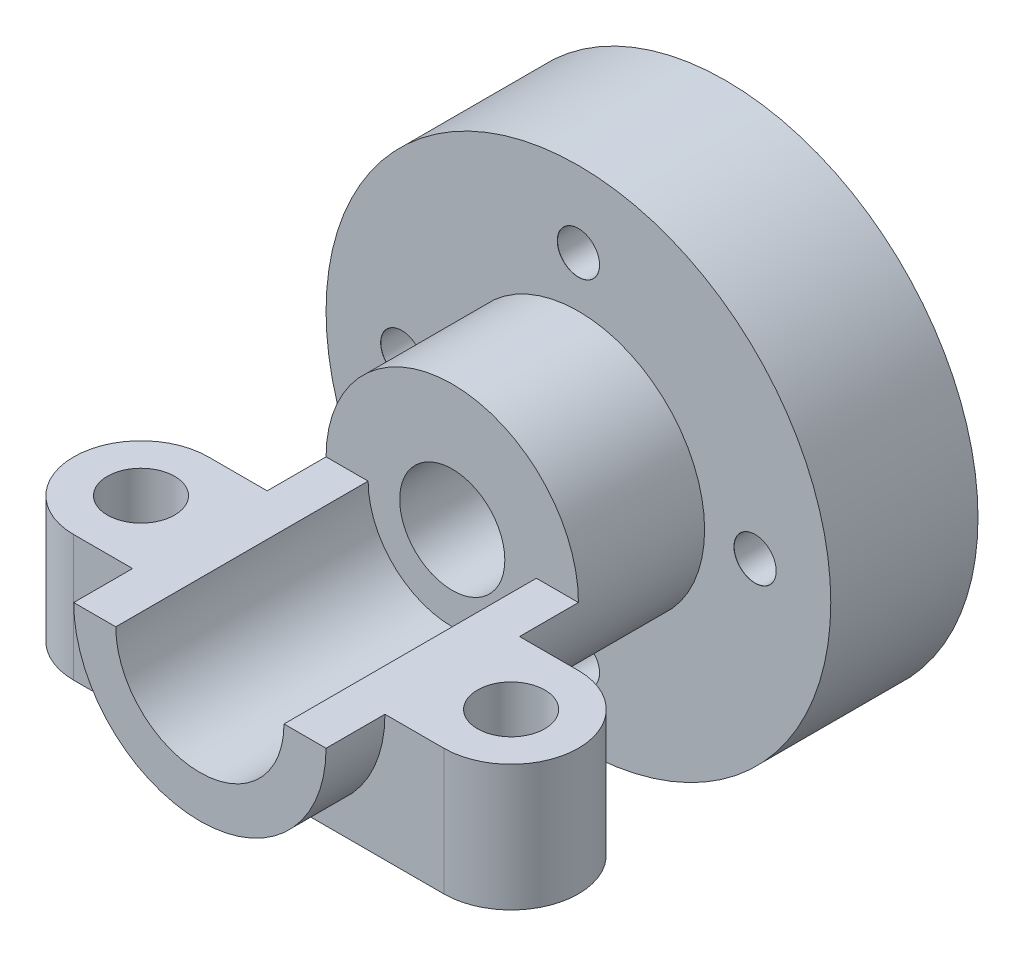
ISO-10303-21;
HEADER;
FILE_DESCRIPTION(('STEP AP214'),'2;1');
FILE_NAME('part.step','',(''),(''),'','','');
FILE_SCHEMA(('AUTOMOTIVE_DESIGN { 1 0 10303 214 1 1 1 1 }'));
ENDSEC;
DATA;
#1=APPLICATION_CONTEXT('core data for automotive mechanical design processes');
#2=APPLICATION_PROTOCOL_DEFINITION('international standard','automotive_design',2000,#1);
#3=PRODUCT_CONTEXT('',#1,'mechanical');
#4=PRODUCT('Part','Part','',(#3));
#5=PRODUCT_RELATED_PRODUCT_CATEGORY('part','',(#4));
#6=PRODUCT_DEFINITION_FORMATION('','',#4);
#7=PRODUCT_DEFINITION_CONTEXT('part definition',#1,'design');
#8=PRODUCT_DEFINITION('design','',#6,#7);
#9=PRODUCT_DEFINITION_SHAPE('','',#8);
#10=(LENGTH_UNIT() NAMED_UNIT(*) SI_UNIT(.MILLI.,.METRE.));
#11=(NAMED_UNIT(*) PLANE_ANGLE_UNIT() SI_UNIT($,.RADIAN.));
#12=(NAMED_UNIT(*) SI_UNIT($,.STERADIAN.) SOLID_ANGLE_UNIT());
#13=UNCERTAINTY_MEASURE_WITH_UNIT(LENGTH_MEASURE(1.E-05),#10,'distance_accuracy_value','');
#14=(GEOMETRIC_REPRESENTATION_CONTEXT(3) GLOBAL_UNCERTAINTY_ASSIGNED_CONTEXT((#13)) GLOBAL_UNIT_ASSIGNED_CONTEXT((#10,
#11,#12)) REPRESENTATION_CONTEXT('',''));
#15=CARTESIAN_POINT('',(0.,0.,0.));
#16=DIRECTION('',(0.,0.,1.));
#17=DIRECTION('',(1.,0.,0.));
#18=AXIS2_PLACEMENT_3D('',#15,#16,#17);
#19=CARTESIAN_POINT('',(-30.,0.,125.));
#20=DIRECTION('',(0.,-1.,0.));
#21=DIRECTION('',(0.,0.,-1.));
#22=AXIS2_PLACEMENT_3D('',#19,#20,#21);
#23=PLANE('',#22);
#24=CARTESIAN_POINT('',(44.,0.,95.));
#25=DIRECTION('',(0.,1.,0.));
#26=DIRECTION('',(0.,0.,1.));
#27=AXIS2_PLACEMENT_3D('',#24,#25,#26);
#28=CIRCLE('',#27,8.);
#29=CARTESIAN_POINT('',(44.,0.,103.));
#30=VERTEX_POINT('',#29);
#31=EDGE_CURVE('E317',#30,#30,#28,.T.);
#32=ORIENTED_EDGE('',*,*,#31,.F.);
#33=EDGE_LOOP('',(#32));
#34=FACE_BOUND('',#33,.T.);
#35=DIRECTION('',(-1.,0.,0.));
#36=VECTOR('',#35,1.);
#37=CARTESIAN_POINT('',(20.,0.,65.));
#38=LINE('',#37,#36);
#39=CARTESIAN_POINT('',(30.,0.,65.));
#40=VERTEX_POINT('',#39);
#41=CARTESIAN_POINT('',(20.,0.,65.));
#42=VERTEX_POINT('',#41);
#43=EDGE_CURVE('E240',#40,#42,#38,.T.);
#44=ORIENTED_EDGE('',*,*,#43,.T.);
#45=DIRECTION('',(0.,0.,-1.));
#46=VECTOR('',#45,1.);
#47=CARTESIAN_POINT('',(20.,0.,125.));
#48=LINE('',#47,#46);
#49=CARTESIAN_POINT('',(20.,0.,125.));
#50=VERTEX_POINT('',#49);
#51=EDGE_CURVE('E63',#50,#42,#48,.T.);
#52=ORIENTED_EDGE('',*,*,#51,.F.);
#53=DIRECTION('',(-1.,0.,0.));
#54=VECTOR('',#53,1.);
#55=CARTESIAN_POINT('',(20.,0.,125.));
#56=LINE('',#55,#54);
#57=CARTESIAN_POINT('',(30.,0.,125.));
#58=VERTEX_POINT('',#57);
#59=EDGE_CURVE('E241',#58,#50,#56,.T.);
#60=ORIENTED_EDGE('',*,*,#59,.F.);
#61=DIRECTION('',(0.,0.,-1.));
#62=VECTOR('',#61,1.);
#63=CARTESIAN_POINT('',(30.,0.,125.));
#64=LINE('',#63,#62);
#65=CARTESIAN_POINT('',(30.,0.,111.));
#66=VERTEX_POINT('',#65);
#67=EDGE_CURVE('E253',#58,#66,#64,.T.);
#68=ORIENTED_EDGE('',*,*,#67,.T.);
#69=DIRECTION('',(1.,0.,0.));
#70=VECTOR('',#69,1.);
#71=CARTESIAN_POINT('',(44.,0.,111.));
#72=LINE('',#71,#70);
#73=CARTESIAN_POINT('',(44.,0.,111.));
#74=VERTEX_POINT('',#73);
#75=EDGE_CURVE('E57',#66,#74,#72,.T.);
#76=ORIENTED_EDGE('',*,*,#75,.T.);
#77=CARTESIAN_POINT('',(44.,0.,95.));
#78=DIRECTION('',(0.,1.,0.));
#79=DIRECTION('',(0.,0.,-1.));
#80=AXIS2_PLACEMENT_3D('',#77,#78,#79);
#81=CIRCLE('',#80,16.);
#82=CARTESIAN_POINT('',(44.,0.,79.));
#83=VERTEX_POINT('',#82);
#84=EDGE_CURVE('E174',#74,#83,#81,.T.);
#85=ORIENTED_EDGE('',*,*,#84,.T.);
#86=DIRECTION('',(-1.,0.,0.));
#87=VECTOR('',#86,1.);
#88=CARTESIAN_POINT('',(-44.,0.,79.));
#89=LINE('',#88,#87);
#90=CARTESIAN_POINT('',(30.,0.,79.));
#91=VERTEX_POINT('',#90);
#92=EDGE_CURVE('E154',#83,#91,#89,.T.);
#93=ORIENTED_EDGE('',*,*,#92,.T.);
#94=EDGE_CURVE('E249',#91,#40,#64,.T.);
#95=ORIENTED_EDGE('',*,*,#94,.T.);
#96=EDGE_LOOP('',(#44,#52,#60,#68,#76,#85,#93,#95));
#97=FACE_BOUND('',#96,.T.);
#98=ADVANCED_FACE('F39',(#34,#97),#23,.F.);
#99=CARTESIAN_POINT('',(0.,0.,65.));
#100=DIRECTION('',(0.,0.,-1.));
#101=DIRECTION('',(-1.,0.,0.));
#102=AXIS2_PLACEMENT_3D('',#99,#100,#101);
#103=CYLINDRICAL_SURFACE('',#102,30.);
#104=DIRECTION('',(0.,0.,-1.));
#105=VECTOR('',#104,1.);
#106=CARTESIAN_POINT('',(-30.,0.,125.));
#107=LINE('',#106,#105);
#108=CARTESIAN_POINT('',(-30.,0.,125.));
#109=VERTEX_POINT('',#108);
#110=CARTESIAN_POINT('',(-30.,0.,111.));
#111=VERTEX_POINT('',#110);
#112=EDGE_CURVE('E254',#109,#111,#107,.T.);
#113=ORIENTED_EDGE('',*,*,#112,.T.);
#114=CARTESIAN_POINT('',(0.,0.,111.));
#115=DIRECTION('',(0.,0.,1.));
#116=DIRECTION('',(1.,0.,0.));
#117=AXIS2_PLACEMENT_3D('',#114,#115,#116);
#118=CIRCLE('',#117,30.);
#119=CARTESIAN_POINT('',(0.,-30.,111.));
#120=VERTEX_POINT('',#119);
#121=EDGE_CURVE('E185',#111,#120,#118,.T.);
#122=ORIENTED_EDGE('',*,*,#121,.T.);
#123=EDGE_CURVE('E180',#120,#66,#118,.T.);
#124=ORIENTED_EDGE('',*,*,#123,.T.);
#125=ORIENTED_EDGE('',*,*,#67,.F.);
#126=CARTESIAN_POINT('',(0.,0.,125.));
#127=DIRECTION('',(0.,0.,1.));
#128=DIRECTION('',(1.,0.,0.));
#129=AXIS2_PLACEMENT_3D('',#126,#127,#128);
#130=CIRCLE('',#129,30.);
#131=EDGE_CURVE('E239',#109,#58,#130,.T.);
#132=ORIENTED_EDGE('',*,*,#131,.F.);
#133=EDGE_LOOP('',(#113,#122,#124,#125,#132));
#134=FACE_BOUND('',#133,.T.);
#135=ADVANCED_FACE('F282',(#134),#103,.T.);
#136=CARTESIAN_POINT('',(0.,0.,-0.001000000000001));
#137=DIRECTION('',(0.,0.,1.));
#138=DIRECTION('',(1.,0.,0.));
#139=AXIS2_PLACEMENT_3D('',#136,#137,#138);
#140=CYLINDRICAL_SURFACE('',#139,12.5);
#141=CARTESIAN_POINT('',(0.,0.,65.));
#142=DIRECTION('',(0.,0.,1.));
#143=DIRECTION('',(1.,0.,0.));
#144=AXIS2_PLACEMENT_3D('',#141,#142,#143);
#145=CIRCLE('',#144,12.5);
#146=CARTESIAN_POINT('',(12.5,0.,65.));
#147=VERTEX_POINT('',#146);
#148=EDGE_CURVE('E228',#147,#147,#145,.T.);
#149=ORIENTED_EDGE('',*,*,#148,.T.);
#150=EDGE_LOOP('',(#149));
#151=FACE_BOUND('',#150,.T.);
#152=CARTESIAN_POINT('',(0.,0.,15.));
#153=DIRECTION('',(0.,0.,-1.));
#154=DIRECTION('',(-1.,0.,0.));
#155=AXIS2_PLACEMENT_3D('',#152,#153,#154);
#156=CIRCLE('',#155,12.5);
#157=CARTESIAN_POINT('',(-12.5,0.,15.));
#158=VERTEX_POINT('',#157);
#159=EDGE_CURVE('E43',#158,#158,#156,.F.);
#160=ORIENTED_EDGE('',*,*,#159,.F.);
#161=EDGE_LOOP('',(#160));
#162=FACE_BOUND('',#161,.T.);
#163=ADVANCED_FACE('F296',(#151,#162),#140,.F.);
#164=CARTESIAN_POINT('',(0.,0.,35.));
#165=DIRECTION('',(0.,0.,-1.));
#166=DIRECTION('',(-1.,0.,0.));
#167=AXIS2_PLACEMENT_3D('',#164,#165,#166);
#168=CYLINDRICAL_SURFACE('',#167,60.);
#169=CARTESIAN_POINT('',(0.,0.,35.));
#170=DIRECTION('',(0.,0.,1.));
#171=DIRECTION('',(1.,0.,0.));
#172=AXIS2_PLACEMENT_3D('',#169,#170,#171);
#173=CIRCLE('',#172,60.);
#174=CARTESIAN_POINT('',(60.,0.,35.));
#175=VERTEX_POINT('',#174);
#176=EDGE_CURVE('E48',#175,#175,#173,.T.);
#177=ORIENTED_EDGE('',*,*,#176,.F.);
#178=EDGE_LOOP('',(#177));
#179=FACE_BOUND('',#178,.T.);
#180=CARTESIAN_POINT('',(0.,0.,0.));
#181=DIRECTION('',(0.,0.,1.));
#182=DIRECTION('',(1.,0.,0.));
#183=AXIS2_PLACEMENT_3D('',#180,#181,#182);
#184=CIRCLE('',#183,60.);
#185=CARTESIAN_POINT('',(60.,0.,0.));
#186=VERTEX_POINT('',#185);
#187=EDGE_CURVE('E265',#186,#186,#184,.T.);
#188=ORIENTED_EDGE('',*,*,#187,.T.);
#189=EDGE_LOOP('',(#188));
#190=FACE_BOUND('',#189,.T.);
#191=ADVANCED_FACE('F41',(#179,#190),#168,.T.);
#192=CARTESIAN_POINT('',(0.,0.,35.));
#193=DIRECTION('',(0.,0.,1.));
#194=DIRECTION('',(1.,0.,0.));
#195=AXIS2_PLACEMENT_3D('',#192,#193,#194);
#196=PLANE('',#195);
#197=CARTESIAN_POINT('',(0.,42.,35.));
#198=DIRECTION('',(0.,0.,1.));
#199=DIRECTION('',(1.,0.,0.));
#200=AXIS2_PLACEMENT_3D('',#197,#198,#199);
#201=CIRCLE('',#200,5.025);
#202=CARTESIAN_POINT('',(5.025,42.,35.));
#203=VERTEX_POINT('',#202);
#204=EDGE_CURVE('E187',#203,#203,#201,.T.);
#205=ORIENTED_EDGE('',*,*,#204,.F.);
#206=EDGE_LOOP('',(#205));
#207=FACE_BOUND('',#206,.T.);
#208=CARTESIAN_POINT('',(42.,0.,35.));
#209=DIRECTION('',(0.,0.,1.));
#210=DIRECTION('',(1.,0.,0.));
#211=AXIS2_PLACEMENT_3D('',#208,#209,#210);
#212=CIRCLE('',#211,5.025);
#213=CARTESIAN_POINT('',(47.025,0.,35.));
#214=VERTEX_POINT('',#213);
#215=EDGE_CURVE('E198',#214,#214,#212,.T.);
#216=ORIENTED_EDGE('',*,*,#215,.F.);
#217=EDGE_LOOP('',(#216));
#218=FACE_BOUND('',#217,.T.);
#219=CARTESIAN_POINT('',(0.,-42.,35.));
#220=DIRECTION('',(0.,0.,1.));
#221=DIRECTION('',(1.,0.,0.));
#222=AXIS2_PLACEMENT_3D('',#219,#220,#221);
#223=CIRCLE('',#222,5.025);
#224=CARTESIAN_POINT('',(5.025,-42.,35.));
#225=VERTEX_POINT('',#224);
#226=EDGE_CURVE('E202',#225,#225,#223,.T.);
#227=ORIENTED_EDGE('',*,*,#226,.F.);
#228=EDGE_LOOP('',(#227));
#229=FACE_BOUND('',#228,.T.);
#230=CARTESIAN_POINT('',(-42.,0.,35.));
#231=DIRECTION('',(0.,0.,1.));
#232=DIRECTION('',(1.,0.,0.));
#233=AXIS2_PLACEMENT_3D('',#230,#231,#232);
#234=CIRCLE('',#233,5.025);
#235=CARTESIAN_POINT('',(-36.975,0.,35.));
#236=VERTEX_POINT('',#235);
#237=EDGE_CURVE('E212',#236,#236,#234,.T.);
#238=ORIENTED_EDGE('',*,*,#237,.F.);
#239=EDGE_LOOP('',(#238));
#240=FACE_BOUND('',#239,.T.);
#241=CARTESIAN_POINT('',(0.,0.,35.));
#242=DIRECTION('',(0.,0.,1.));
#243=DIRECTION('',(1.,0.,0.));
#244=AXIS2_PLACEMENT_3D('',#241,#242,#243);
#245=CIRCLE('',#244,30.);
#246=CARTESIAN_POINT('',(30.,0.,35.));
#247=VERTEX_POINT('',#246);
#248=EDGE_CURVE('E11',#247,#247,#245,.T.);
#249=ORIENTED_EDGE('',*,*,#248,.F.);
#250=EDGE_LOOP('',(#249));
#251=FACE_BOUND('',#250,.T.);
#252=ORIENTED_EDGE('',*,*,#176,.T.);
#253=EDGE_LOOP('',(#252));
#254=FACE_BOUND('',#253,.T.);
#255=ADVANCED_FACE('F275',(#207,#218,#229,#240,#251,#254),#196,.T.);
#256=CARTESIAN_POINT('',(0.,0.,0.));
#257=DIRECTION('',(0.,0.,1.));
#258=DIRECTION('',(1.,0.,0.));
#259=AXIS2_PLACEMENT_3D('',#256,#257,#258);
#260=PLANE('',#259);
#261=CARTESIAN_POINT('',(0.,0.,0.));
#262=DIRECTION('',(0.,0.,-1.));
#263=DIRECTION('',(-1.,0.,0.));
#264=AXIS2_PLACEMENT_3D('',#261,#262,#263);
#265=CIRCLE('',#264,55.);
#266=CARTESIAN_POINT('',(-55.,0.,0.));
#267=VERTEX_POINT('',#266);
#268=EDGE_CURVE('E224',#267,#267,#265,.T.);
#269=ORIENTED_EDGE('',*,*,#268,.F.);
#270=EDGE_LOOP('',(#269));
#271=FACE_BOUND('',#270,.T.);
#272=ORIENTED_EDGE('',*,*,#187,.F.);
#273=EDGE_LOOP('',(#272));
#274=FACE_BOUND('',#273,.T.);
#275=ADVANCED_FACE('F267',(#271,#274),#260,.F.);
#276=ORIENTED_EDGE('',*,*,#94,.F.);
#277=CARTESIAN_POINT('',(0.,0.,79.));
#278=DIRECTION('',(0.,0.,-1.));
#279=DIRECTION('',(-1.,0.,0.));
#280=AXIS2_PLACEMENT_3D('',#277,#278,#279);
#281=CIRCLE('',#280,30.);
#282=CARTESIAN_POINT('',(0.,-30.,79.));
#283=VERTEX_POINT('',#282);
#284=EDGE_CURVE('E186',#91,#283,#281,.T.);
#285=ORIENTED_EDGE('',*,*,#284,.T.);
#286=CARTESIAN_POINT('',(-30.,0.,79.));
#287=VERTEX_POINT('',#286);
#288=EDGE_CURVE('E181',#283,#287,#281,.T.);
#289=ORIENTED_EDGE('',*,*,#288,.T.);
#290=CARTESIAN_POINT('',(-30.,0.,65.));
#291=VERTEX_POINT('',#290);
#292=EDGE_CURVE('E255',#287,#291,#107,.T.);
#293=ORIENTED_EDGE('',*,*,#292,.T.);
#294=CARTESIAN_POINT('',(0.,0.,65.));
#295=DIRECTION('',(0.,0.,1.));
#296=DIRECTION('',(1.,0.,0.));
#297=AXIS2_PLACEMENT_3D('',#294,#295,#296);
#298=CIRCLE('',#297,30.);
#299=EDGE_CURVE('E257',#40,#291,#298,.T.);
#300=ORIENTED_EDGE('',*,*,#299,.F.);
#301=EDGE_LOOP('',(#276,#285,#289,#293,#300));
#302=FACE_BOUND('',#301,.T.);
#303=ORIENTED_EDGE('',*,*,#248,.T.);
#304=EDGE_LOOP('',(#303));
#305=FACE_BOUND('',#304,.T.);
#306=ADVANCED_FACE('F271',(#302,#305),#103,.T.);
#307=CARTESIAN_POINT('',(0.,0.,65.));
#308=DIRECTION('',(0.,0.,1.));
#309=DIRECTION('',(1.,0.,0.));
#310=AXIS2_PLACEMENT_3D('',#307,#308,#309);
#311=PLANE('',#310);
#312=ORIENTED_EDGE('',*,*,#148,.F.);
#313=EDGE_LOOP('',(#312));
#314=FACE_BOUND('',#313,.T.);
#315=ORIENTED_EDGE('',*,*,#43,.F.);
#316=ORIENTED_EDGE('',*,*,#299,.T.);
#317=DIRECTION('',(-1.,0.,0.));
#318=VECTOR('',#317,1.);
#319=CARTESIAN_POINT('',(-30.,0.,65.));
#320=LINE('',#319,#318);
#321=CARTESIAN_POINT('',(-20.,0.,65.));
#322=VERTEX_POINT('',#321);
#323=EDGE_CURVE('E243',#322,#291,#320,.T.);
#324=ORIENTED_EDGE('',*,*,#323,.F.);
#325=CARTESIAN_POINT('',(0.,0.,65.));
#326=DIRECTION('',(0.,0.,-1.));
#327=DIRECTION('',(1.,0.,0.));
#328=AXIS2_PLACEMENT_3D('',#325,#326,#327);
#329=CIRCLE('',#328,20.);
#330=EDGE_CURVE('E235',#42,#322,#329,.T.);
#331=ORIENTED_EDGE('',*,*,#330,.F.);
#332=EDGE_LOOP('',(#315,#316,#324,#331));
#333=FACE_BOUND('',#332,.T.);
#334=ADVANCED_FACE('F276',(#314,#333),#311,.T.);
#335=CARTESIAN_POINT('',(0.,0.,125.));
#336=DIRECTION('',(0.,0.,-1.));
#337=DIRECTION('',(-1.,0.,0.));
#338=AXIS2_PLACEMENT_3D('',#335,#336,#337);
#339=CYLINDRICAL_SURFACE('',#338,20.);
#340=ORIENTED_EDGE('',*,*,#51,.T.);
#341=ORIENTED_EDGE('',*,*,#330,.T.);
#342=DIRECTION('',(0.,0.,-1.));
#343=VECTOR('',#342,1.);
#344=CARTESIAN_POINT('',(-20.,0.,125.));
#345=LINE('',#344,#343);
#346=CARTESIAN_POINT('',(-20.,0.,125.));
#347=VERTEX_POINT('',#346);
#348=EDGE_CURVE('E256',#347,#322,#345,.T.);
#349=ORIENTED_EDGE('',*,*,#348,.F.);
#350=CARTESIAN_POINT('',(0.,0.,125.));
#351=DIRECTION('',(0.,0.,-1.));
#352=DIRECTION('',(1.,0.,0.));
#353=AXIS2_PLACEMENT_3D('',#350,#351,#352);
#354=CIRCLE('',#353,20.);
#355=EDGE_CURVE('E231',#50,#347,#354,.T.);
#356=ORIENTED_EDGE('',*,*,#355,.F.);
#357=EDGE_LOOP('',(#340,#341,#349,#356));
#358=FACE_BOUND('',#357,.T.);
#359=ADVANCED_FACE('F302',(#358),#339,.F.);
#360=ORIENTED_EDGE('',*,*,#292,.F.);
#361=CARTESIAN_POINT('',(-44.,0.,79.));
#362=VERTEX_POINT('',#361);
#363=EDGE_CURVE('E158',#287,#362,#89,.T.);
#364=ORIENTED_EDGE('',*,*,#363,.T.);
#365=CARTESIAN_POINT('',(-44.,0.,95.));
#366=DIRECTION('',(0.,1.,0.));
#367=DIRECTION('',(0.,0.,1.));
#368=AXIS2_PLACEMENT_3D('',#365,#366,#367);
#369=CIRCLE('',#368,16.);
#370=CARTESIAN_POINT('',(-44.,0.,111.));
#371=VERTEX_POINT('',#370);
#372=EDGE_CURVE('E166',#362,#371,#369,.T.);
#373=ORIENTED_EDGE('',*,*,#372,.T.);
#374=EDGE_CURVE('E132',#371,#111,#72,.T.);
#375=ORIENTED_EDGE('',*,*,#374,.T.);
#376=ORIENTED_EDGE('',*,*,#112,.F.);
#377=DIRECTION('',(-1.,0.,0.));
#378=VECTOR('',#377,1.);
#379=CARTESIAN_POINT('',(-30.,0.,125.));
#380=LINE('',#379,#378);
#381=EDGE_CURVE('E237',#347,#109,#380,.T.);
#382=ORIENTED_EDGE('',*,*,#381,.F.);
#383=ORIENTED_EDGE('',*,*,#348,.T.);
#384=ORIENTED_EDGE('',*,*,#323,.T.);
#385=EDGE_LOOP('',(#360,#364,#373,#375,#376,#382,#383,#384));
#386=FACE_BOUND('',#385,.T.);
#387=CARTESIAN_POINT('',(-44.,0.,95.));
#388=DIRECTION('',(0.,1.,0.));
#389=DIRECTION('',(0.,0.,1.));
#390=AXIS2_PLACEMENT_3D('',#387,#388,#389);
#391=CIRCLE('',#390,8.);
#392=CARTESIAN_POINT('',(-44.,0.,103.));
#393=VERTEX_POINT('',#392);
#394=EDGE_CURVE('E161',#393,#393,#391,.T.);
#395=ORIENTED_EDGE('',*,*,#394,.F.);
#396=EDGE_LOOP('',(#395));
#397=FACE_BOUND('',#396,.T.);
#398=ADVANCED_FACE('F289',(#386,#397),#23,.F.);
#399=CARTESIAN_POINT('',(0.,0.,125.));
#400=DIRECTION('',(0.,0.,1.));
#401=DIRECTION('',(1.,0.,0.));
#402=AXIS2_PLACEMENT_3D('',#399,#400,#401);
#403=PLANE('',#402);
#404=ORIENTED_EDGE('',*,*,#355,.T.);
#405=ORIENTED_EDGE('',*,*,#381,.T.);
#406=ORIENTED_EDGE('',*,*,#131,.T.);
#407=ORIENTED_EDGE('',*,*,#59,.T.);
#408=EDGE_LOOP('',(#404,#405,#406,#407));
#409=FACE_BOUND('',#408,.T.);
#410=ADVANCED_FACE('F301',(#409),#403,.T.);
#411=CARTESIAN_POINT('',(0.,0.,15.));
#412=DIRECTION('',(0.,0.,-1.));
#413=DIRECTION('',(-1.,0.,0.));
#414=AXIS2_PLACEMENT_3D('',#411,#412,#413);
#415=PLANE('',#414);
#416=CARTESIAN_POINT('',(0.,42.,15.));
#417=DIRECTION('',(0.,0.,-1.));
#418=DIRECTION('',(-1.,0.,0.));
#419=AXIS2_PLACEMENT_3D('',#416,#417,#418);
#420=CIRCLE('',#419,5.);
#421=CARTESIAN_POINT('',(-5.,42.,15.));
#422=VERTEX_POINT('',#421);
#423=EDGE_CURVE('E191',#422,#422,#420,.T.);
#424=ORIENTED_EDGE('',*,*,#423,.F.);
#425=EDGE_LOOP('',(#424));
#426=FACE_BOUND('',#425,.T.);
#427=CARTESIAN_POINT('',(42.,0.,15.));
#428=DIRECTION('',(0.,0.,-1.));
#429=DIRECTION('',(-1.,0.,0.));
#430=AXIS2_PLACEMENT_3D('',#427,#428,#429);
#431=CIRCLE('',#430,5.);
#432=CARTESIAN_POINT('',(37.,0.,15.));
#433=VERTEX_POINT('',#432);
#434=EDGE_CURVE('E205',#433,#433,#431,.T.);
#435=ORIENTED_EDGE('',*,*,#434,.F.);
#436=EDGE_LOOP('',(#435));
#437=FACE_BOUND('',#436,.T.);
#438=CARTESIAN_POINT('',(0.,-42.,15.));
#439=DIRECTION('',(0.,0.,-1.));
#440=DIRECTION('',(-1.,0.,0.));
#441=AXIS2_PLACEMENT_3D('',#438,#439,#440);
#442=CIRCLE('',#441,5.);
#443=CARTESIAN_POINT('',(-5.,-42.,15.));
#444=VERTEX_POINT('',#443);
#445=EDGE_CURVE('E211',#444,#444,#442,.T.);
#446=ORIENTED_EDGE('',*,*,#445,.F.);
#447=EDGE_LOOP('',(#446));
#448=FACE_BOUND('',#447,.T.);
#449=CARTESIAN_POINT('',(-42.,0.,15.));
#450=DIRECTION('',(0.,0.,-1.));
#451=DIRECTION('',(-1.,0.,0.));
#452=AXIS2_PLACEMENT_3D('',#449,#450,#451);
#453=CIRCLE('',#452,5.);
#454=CARTESIAN_POINT('',(-47.,0.,15.));
#455=VERTEX_POINT('',#454);
#456=EDGE_CURVE('E219',#455,#455,#453,.T.);
#457=ORIENTED_EDGE('',*,*,#456,.F.);
#458=EDGE_LOOP('',(#457));
#459=FACE_BOUND('',#458,.T.);
#460=CARTESIAN_POINT('',(0.,0.,15.));
#461=DIRECTION('',(0.,0.,-1.));
#462=DIRECTION('',(-1.,0.,0.));
#463=AXIS2_PLACEMENT_3D('',#460,#461,#462);
#464=CIRCLE('',#463,55.);
#465=CARTESIAN_POINT('',(-55.,0.,15.));
#466=VERTEX_POINT('',#465);
#467=EDGE_CURVE('E221',#466,#466,#464,.T.);
#468=ORIENTED_EDGE('',*,*,#467,.T.);
#469=EDGE_LOOP('',(#468));
#470=FACE_BOUND('',#469,.T.);
#471=ORIENTED_EDGE('',*,*,#159,.T.);
#472=EDGE_LOOP('',(#471));
#473=FACE_BOUND('',#472,.T.);
#474=ADVANCED_FACE('F310',(#426,#437,#448,#459,#470,#473),#415,.T.);
#475=CARTESIAN_POINT('',(0.,0.,15.));
#476=DIRECTION('',(0.,0.,-1.));
#477=DIRECTION('',(-1.,0.,0.));
#478=AXIS2_PLACEMENT_3D('',#475,#476,#477);
#479=CYLINDRICAL_SURFACE('',#478,55.);
#480=ORIENTED_EDGE('',*,*,#467,.F.);
#481=EDGE_LOOP('',(#480));
#482=FACE_BOUND('',#481,.T.);
#483=ORIENTED_EDGE('',*,*,#268,.T.);
#484=EDGE_LOOP('',(#483));
#485=FACE_BOUND('',#484,.T.);
#486=ADVANCED_FACE('F382',(#482,#485),#479,.F.);
#487=CARTESIAN_POINT('',(-42.,0.,35.));
#488=DIRECTION('',(0.,0.,1.));
#489=DIRECTION('',(1.,0.,0.));
#490=AXIS2_PLACEMENT_3D('',#487,#488,#489);
#491=CYLINDRICAL_SURFACE('',#490,5.);
#492=CARTESIAN_POINT('',(-42.,0.,34.975));
#493=DIRECTION('',(0.,0.,1.));
#494=DIRECTION('',(1.,0.,0.));
#495=AXIS2_PLACEMENT_3D('',#492,#493,#494);
#496=CIRCLE('',#495,5.);
#497=CARTESIAN_POINT('',(-37.,0.,34.975));
#498=VERTEX_POINT('',#497);
#499=EDGE_CURVE('E220',#498,#498,#496,.T.);
#500=ORIENTED_EDGE('',*,*,#499,.T.);
#501=EDGE_LOOP('',(#500));
#502=FACE_BOUND('',#501,.T.);
#503=ORIENTED_EDGE('',*,*,#456,.T.);
#504=EDGE_LOOP('',(#503));
#505=FACE_BOUND('',#504,.T.);
#506=ADVANCED_FACE('F377',(#502,#505),#491,.F.);
#507=CARTESIAN_POINT('',(-42.,0.,35.));
#508=DIRECTION('',(0.,0.,1.));
#509=DIRECTION('',(1.,0.,0.));
#510=AXIS2_PLACEMENT_3D('',#507,#508,#509);
#511=CONICAL_SURFACE('',#510,5.025,0.785398163397587);
#512=ORIENTED_EDGE('',*,*,#499,.F.);
#513=EDGE_LOOP('',(#512));
#514=FACE_BOUND('',#513,.T.);
#515=ORIENTED_EDGE('',*,*,#237,.T.);
#516=EDGE_LOOP('',(#515));
#517=FACE_BOUND('',#516,.T.);
#518=ADVANCED_FACE('F374',(#514,#517),#511,.F.);
#519=CARTESIAN_POINT('',(0.,-42.,35.));
#520=DIRECTION('',(0.,0.,1.));
#521=DIRECTION('',(1.,0.,0.));
#522=AXIS2_PLACEMENT_3D('',#519,#520,#521);
#523=CYLINDRICAL_SURFACE('',#522,5.);
#524=CARTESIAN_POINT('',(0.,-42.,34.975));
#525=DIRECTION('',(0.,0.,1.));
#526=DIRECTION('',(1.,0.,0.));
#527=AXIS2_PLACEMENT_3D('',#524,#525,#526);
#528=CIRCLE('',#527,5.);
#529=CARTESIAN_POINT('',(5.,-42.,34.975));
#530=VERTEX_POINT('',#529);
#531=EDGE_CURVE('E208',#530,#530,#528,.T.);
#532=ORIENTED_EDGE('',*,*,#531,.T.);
#533=EDGE_LOOP('',(#532));
#534=FACE_BOUND('',#533,.T.);
#535=ORIENTED_EDGE('',*,*,#445,.T.);
#536=EDGE_LOOP('',(#535));
#537=FACE_BOUND('',#536,.T.);
#538=ADVANCED_FACE('F371',(#534,#537),#523,.F.);
#539=CARTESIAN_POINT('',(0.,-42.,35.));
#540=DIRECTION('',(0.,0.,1.));
#541=DIRECTION('',(1.,0.,0.));
#542=AXIS2_PLACEMENT_3D('',#539,#540,#541);
#543=CONICAL_SURFACE('',#542,5.025,0.785398163397535);
#544=ORIENTED_EDGE('',*,*,#531,.F.);
#545=EDGE_LOOP('',(#544));
#546=FACE_BOUND('',#545,.T.);
#547=ORIENTED_EDGE('',*,*,#226,.T.);
#548=EDGE_LOOP('',(#547));
#549=FACE_BOUND('',#548,.T.);
#550=ADVANCED_FACE('F370',(#546,#549),#543,.F.);
#551=CARTESIAN_POINT('',(42.,0.,35.));
#552=DIRECTION('',(0.,0.,1.));
#553=DIRECTION('',(1.,0.,0.));
#554=AXIS2_PLACEMENT_3D('',#551,#552,#553);
#555=CYLINDRICAL_SURFACE('',#554,5.);
#556=CARTESIAN_POINT('',(42.,0.,34.975));
#557=DIRECTION('',(0.,0.,1.));
#558=DIRECTION('',(1.,0.,0.));
#559=AXIS2_PLACEMENT_3D('',#556,#557,#558);
#560=CIRCLE('',#559,5.);
#561=CARTESIAN_POINT('',(47.,0.,34.975));
#562=VERTEX_POINT('',#561);
#563=EDGE_CURVE('E200',#562,#562,#560,.T.);
#564=ORIENTED_EDGE('',*,*,#563,.T.);
#565=EDGE_LOOP('',(#564));
#566=FACE_BOUND('',#565,.T.);
#567=ORIENTED_EDGE('',*,*,#434,.T.);
#568=EDGE_LOOP('',(#567));
#569=FACE_BOUND('',#568,.T.);
#570=ADVANCED_FACE('F361',(#566,#569),#555,.F.);
#571=CARTESIAN_POINT('',(42.,0.,35.));
#572=DIRECTION('',(0.,0.,1.));
#573=DIRECTION('',(1.,0.,0.));
#574=AXIS2_PLACEMENT_3D('',#571,#572,#573);
#575=CONICAL_SURFACE('',#574,5.025,0.785398163397587);
#576=ORIENTED_EDGE('',*,*,#563,.F.);
#577=EDGE_LOOP('',(#576));
#578=FACE_BOUND('',#577,.T.);
#579=ORIENTED_EDGE('',*,*,#215,.T.);
#580=EDGE_LOOP('',(#579));
#581=FACE_BOUND('',#580,.T.);
#582=ADVANCED_FACE('F357',(#578,#581),#575,.F.);
#583=CARTESIAN_POINT('',(0.,42.,35.));
#584=DIRECTION('',(0.,0.,1.));
#585=DIRECTION('',(1.,0.,0.));
#586=AXIS2_PLACEMENT_3D('',#583,#584,#585);
#587=CYLINDRICAL_SURFACE('',#586,5.);
#588=CARTESIAN_POINT('',(0.,42.,34.975));
#589=DIRECTION('',(0.,0.,1.));
#590=DIRECTION('',(1.,0.,0.));
#591=AXIS2_PLACEMENT_3D('',#588,#589,#590);
#592=CIRCLE('',#591,5.);
#593=CARTESIAN_POINT('',(5.,42.,34.975));
#594=VERTEX_POINT('',#593);
#595=EDGE_CURVE('E190',#594,#594,#592,.T.);
#596=ORIENTED_EDGE('',*,*,#595,.T.);
#597=EDGE_LOOP('',(#596));
#598=FACE_BOUND('',#597,.T.);
#599=ORIENTED_EDGE('',*,*,#423,.T.);
#600=EDGE_LOOP('',(#599));
#601=FACE_BOUND('',#600,.T.);
#602=ADVANCED_FACE('F355',(#598,#601),#587,.F.);
#603=CARTESIAN_POINT('',(0.,42.,35.));
#604=DIRECTION('',(0.,0.,1.));
#605=DIRECTION('',(1.,0.,0.));
#606=AXIS2_PLACEMENT_3D('',#603,#604,#605);
#607=CONICAL_SURFACE('',#606,5.025,0.785398163397535);
#608=ORIENTED_EDGE('',*,*,#595,.F.);
#609=EDGE_LOOP('',(#608));
#610=FACE_BOUND('',#609,.T.);
#611=ORIENTED_EDGE('',*,*,#204,.T.);
#612=EDGE_LOOP('',(#611));
#613=FACE_BOUND('',#612,.T.);
#614=ADVANCED_FACE('F340',(#610,#613),#607,.F.);
#615=CARTESIAN_POINT('',(-44.,-30.,95.));
#616=DIRECTION('',(0.,1.,0.));
#617=DIRECTION('',(0.,0.,1.));
#618=AXIS2_PLACEMENT_3D('',#615,#616,#617);
#619=PLANE('',#618);
#620=CARTESIAN_POINT('',(44.,-30.,95.));
#621=DIRECTION('',(0.,1.,0.));
#622=DIRECTION('',(0.,0.,1.));
#623=AXIS2_PLACEMENT_3D('',#620,#621,#622);
#624=CIRCLE('',#623,8.);
#625=CARTESIAN_POINT('',(44.,-30.,103.));
#626=VERTEX_POINT('',#625);
#627=EDGE_CURVE('E316',#626,#626,#624,.T.);
#628=ORIENTED_EDGE('',*,*,#627,.T.);
#629=EDGE_LOOP('',(#628));
#630=FACE_BOUND('',#629,.T.);
#631=DIRECTION('',(1.,0.,0.));
#632=VECTOR('',#631,1.);
#633=CARTESIAN_POINT('',(44.,-30.,111.));
#634=LINE('',#633,#632);
#635=CARTESIAN_POINT('',(44.,-30.,111.));
#636=VERTEX_POINT('',#635);
#637=EDGE_CURVE('E146',#120,#636,#634,.T.);
#638=ORIENTED_EDGE('',*,*,#637,.F.);
#639=CARTESIAN_POINT('',(-44.,-30.,111.));
#640=VERTEX_POINT('',#639);
#641=EDGE_CURVE('E129',#640,#120,#634,.T.);
#642=ORIENTED_EDGE('',*,*,#641,.F.);
#643=CARTESIAN_POINT('',(-44.,-30.,95.));
#644=DIRECTION('',(0.,1.,0.));
#645=DIRECTION('',(0.,0.,1.));
#646=AXIS2_PLACEMENT_3D('',#643,#644,#645);
#647=CIRCLE('',#646,16.);
#648=CARTESIAN_POINT('',(-44.,-30.,79.));
#649=VERTEX_POINT('',#648);
#650=EDGE_CURVE('E148',#649,#640,#647,.T.);
#651=ORIENTED_EDGE('',*,*,#650,.F.);
#652=DIRECTION('',(-1.,0.,0.));
#653=VECTOR('',#652,1.);
#654=CARTESIAN_POINT('',(-44.,-30.,79.));
#655=LINE('',#654,#653);
#656=EDGE_CURVE('E167',#283,#649,#655,.T.);
#657=ORIENTED_EDGE('',*,*,#656,.F.);
#658=CARTESIAN_POINT('',(44.,-30.,79.));
#659=VERTEX_POINT('',#658);
#660=EDGE_CURVE('E136',#659,#283,#655,.T.);
#661=ORIENTED_EDGE('',*,*,#660,.F.);
#662=CARTESIAN_POINT('',(44.,-30.,95.));
#663=DIRECTION('',(0.,1.,0.));
#664=DIRECTION('',(0.,0.,-1.));
#665=AXIS2_PLACEMENT_3D('',#662,#663,#664);
#666=CIRCLE('',#665,16.);
#667=EDGE_CURVE('E149',#636,#659,#666,.T.);
#668=ORIENTED_EDGE('',*,*,#667,.F.);
#669=EDGE_LOOP('',(#638,#642,#651,#657,#661,#668));
#670=FACE_BOUND('',#669,.T.);
#671=CARTESIAN_POINT('',(-44.,-30.,95.));
#672=DIRECTION('',(0.,1.,0.));
#673=DIRECTION('',(0.,0.,1.));
#674=AXIS2_PLACEMENT_3D('',#671,#672,#673);
#675=CIRCLE('',#674,8.);
#676=CARTESIAN_POINT('',(-44.,-30.,103.));
#677=VERTEX_POINT('',#676);
#678=EDGE_CURVE('E171',#677,#677,#675,.T.);
#679=ORIENTED_EDGE('',*,*,#678,.T.);
#680=EDGE_LOOP('',(#679));
#681=FACE_BOUND('',#680,.T.);
#682=ADVANCED_FACE('F141',(#630,#670,#681),#619,.F.);
#683=CARTESIAN_POINT('',(-44.,-30.,79.));
#684=DIRECTION('',(0.,0.,-1.));
#685=DIRECTION('',(-1.,0.,0.));
#686=AXIS2_PLACEMENT_3D('',#683,#684,#685);
#687=PLANE('',#686);
#688=ORIENTED_EDGE('',*,*,#284,.F.);
#689=ORIENTED_EDGE('',*,*,#92,.F.);
#690=DIRECTION('',(0.,1.,0.));
#691=VECTOR('',#690,1.);
#692=CARTESIAN_POINT('',(44.,-30.,79.));
#693=LINE('',#692,#691);
#694=EDGE_CURVE('E176',#659,#83,#693,.T.);
#695=ORIENTED_EDGE('',*,*,#694,.F.);
#696=ORIENTED_EDGE('',*,*,#660,.T.);
#697=EDGE_LOOP('',(#688,#689,#695,#696));
#698=FACE_BOUND('',#697,.T.);
#699=ADVANCED_FACE('F338',(#698),#687,.T.);
#700=ORIENTED_EDGE('',*,*,#288,.F.);
#701=ORIENTED_EDGE('',*,*,#656,.T.);
#702=DIRECTION('',(0.,1.,0.));
#703=VECTOR('',#702,1.);
#704=CARTESIAN_POINT('',(-44.,-30.,79.));
#705=LINE('',#704,#703);
#706=EDGE_CURVE('E152',#649,#362,#705,.T.);
#707=ORIENTED_EDGE('',*,*,#706,.T.);
#708=ORIENTED_EDGE('',*,*,#363,.F.);
#709=EDGE_LOOP('',(#700,#701,#707,#708));
#710=FACE_BOUND('',#709,.T.);
#711=ADVANCED_FACE('F341',(#710),#687,.T.);
#712=CARTESIAN_POINT('',(44.,-30.,111.));
#713=DIRECTION('',(0.,0.,1.));
#714=DIRECTION('',(1.,0.,0.));
#715=AXIS2_PLACEMENT_3D('',#712,#713,#714);
#716=PLANE('',#715);
#717=ORIENTED_EDGE('',*,*,#121,.F.);
#718=ORIENTED_EDGE('',*,*,#374,.F.);
#719=DIRECTION('',(0.,1.,0.));
#720=VECTOR('',#719,1.);
#721=CARTESIAN_POINT('',(-44.,-30.,111.));
#722=LINE('',#721,#720);
#723=EDGE_CURVE('E127',#640,#371,#722,.T.);
#724=ORIENTED_EDGE('',*,*,#723,.F.);
#725=ORIENTED_EDGE('',*,*,#641,.T.);
#726=EDGE_LOOP('',(#717,#718,#724,#725));
#727=FACE_BOUND('',#726,.T.);
#728=ADVANCED_FACE('F126',(#727),#716,.T.);
#729=ORIENTED_EDGE('',*,*,#123,.F.);
#730=ORIENTED_EDGE('',*,*,#637,.T.);
#731=DIRECTION('',(0.,1.,0.));
#732=VECTOR('',#731,1.);
#733=CARTESIAN_POINT('',(44.,-30.,111.));
#734=LINE('',#733,#732);
#735=EDGE_CURVE('E140',#636,#74,#734,.T.);
#736=ORIENTED_EDGE('',*,*,#735,.T.);
#737=ORIENTED_EDGE('',*,*,#75,.F.);
#738=EDGE_LOOP('',(#729,#730,#736,#737));
#739=FACE_BOUND('',#738,.T.);
#740=ADVANCED_FACE('F348',(#739),#716,.T.);
#741=CARTESIAN_POINT('',(-44.,-30.,95.));
#742=DIRECTION('',(0.,1.,0.));
#743=DIRECTION('',(0.,0.,1.));
#744=AXIS2_PLACEMENT_3D('',#741,#742,#743);
#745=CYLINDRICAL_SURFACE('',#744,16.);
#746=ORIENTED_EDGE('',*,*,#372,.F.);
#747=ORIENTED_EDGE('',*,*,#706,.F.);
#748=ORIENTED_EDGE('',*,*,#650,.T.);
#749=ORIENTED_EDGE('',*,*,#723,.T.);
#750=EDGE_LOOP('',(#746,#747,#748,#749));
#751=FACE_BOUND('',#750,.T.);
#752=ADVANCED_FACE('F155',(#751),#745,.T.);
#753=CARTESIAN_POINT('',(44.,-30.,95.));
#754=DIRECTION('',(0.,1.,0.));
#755=DIRECTION('',(0.,0.,1.));
#756=AXIS2_PLACEMENT_3D('',#753,#754,#755);
#757=CYLINDRICAL_SURFACE('',#756,16.);
#758=ORIENTED_EDGE('',*,*,#84,.F.);
#759=ORIENTED_EDGE('',*,*,#735,.F.);
#760=ORIENTED_EDGE('',*,*,#667,.T.);
#761=ORIENTED_EDGE('',*,*,#694,.T.);
#762=EDGE_LOOP('',(#758,#759,#760,#761));
#763=FACE_BOUND('',#762,.T.);
#764=ADVANCED_FACE('F334',(#763),#757,.T.);
#765=CARTESIAN_POINT('',(-44.,-30.,95.));
#766=DIRECTION('',(0.,1.,0.));
#767=DIRECTION('',(0.,0.,1.));
#768=AXIS2_PLACEMENT_3D('',#765,#766,#767);
#769=CYLINDRICAL_SURFACE('',#768,8.);
#770=ORIENTED_EDGE('',*,*,#678,.F.);
#771=EDGE_LOOP('',(#770));
#772=FACE_BOUND('',#771,.T.);
#773=ORIENTED_EDGE('',*,*,#394,.T.);
#774=EDGE_LOOP('',(#773));
#775=FACE_BOUND('',#774,.T.);
#776=ADVANCED_FACE('F330',(#772,#775),#769,.F.);
#777=CARTESIAN_POINT('',(44.,-30.,95.));
#778=DIRECTION('',(0.,1.,0.));
#779=DIRECTION('',(0.,0.,1.));
#780=AXIS2_PLACEMENT_3D('',#777,#778,#779);
#781=CYLINDRICAL_SURFACE('',#780,8.);
#782=ORIENTED_EDGE('',*,*,#627,.F.);
#783=EDGE_LOOP('',(#782));
#784=FACE_BOUND('',#783,.T.);
#785=ORIENTED_EDGE('',*,*,#31,.T.);
#786=EDGE_LOOP('',(#785));
#787=FACE_BOUND('',#786,.T.);
#788=ADVANCED_FACE('F326',(#784,#787),#781,.F.);
#789=CLOSED_SHELL('',(#98,#135,#163,#191,#255,#275,#306,#334,#359,#398,#410,#474,#486,#506,#518,
#538,#550,#570,#582,#602,#614,#682,#699,#711,#728,#740,#752,#764,#776,#788));
#790=MANIFOLD_SOLID_BREP('B2',#789);
#791=ADVANCED_BREP_SHAPE_REPRESENTATION('',(#18,#790),#14);
#792=SHAPE_DEFINITION_REPRESENTATION(#9,#791);
ENDSEC;
END-ISO-10303-21;
